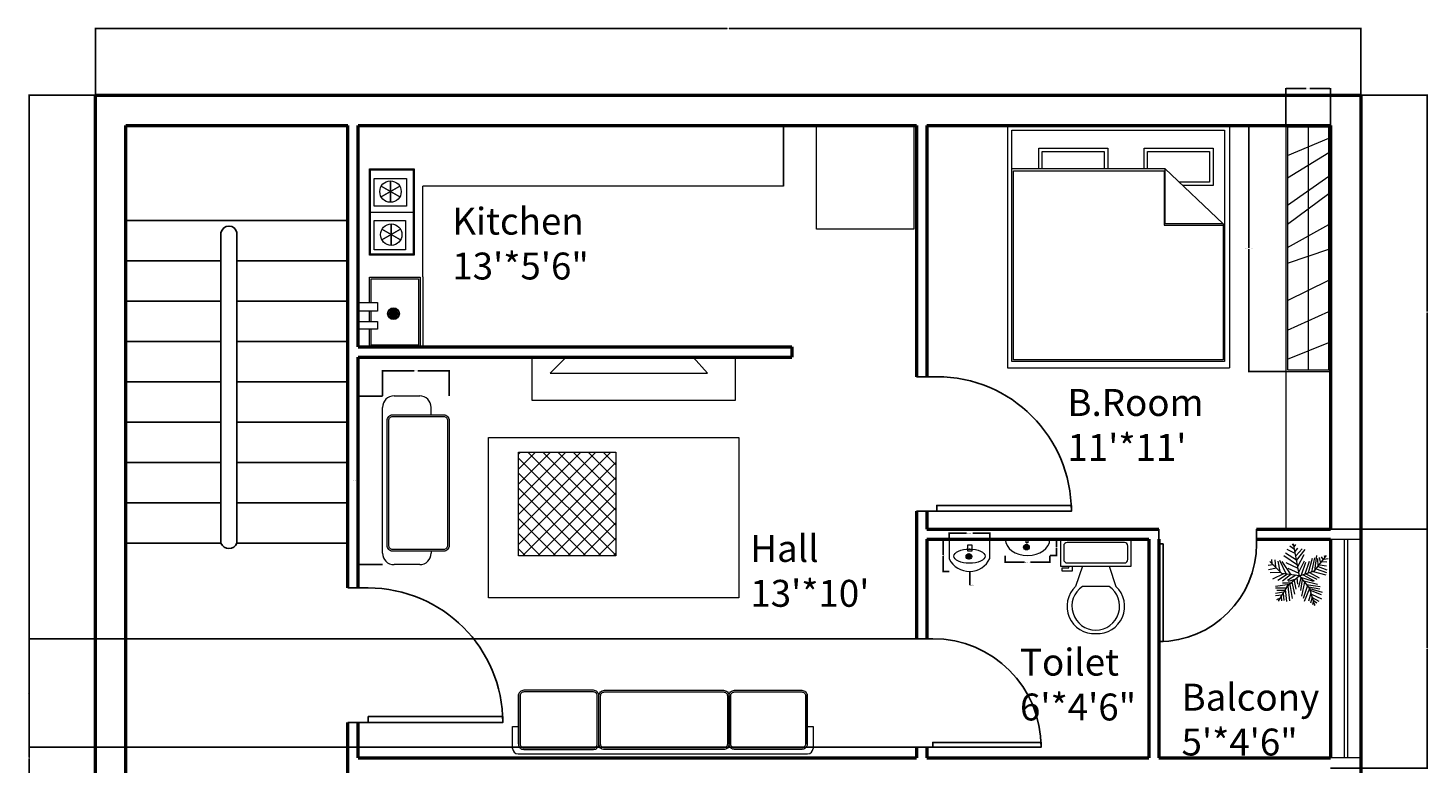
# Model space of a CAD drawing. Units: inches. Extents: x 132738 to 133154, y 138207 to 138641.
# Tile 2 of 2: x 132738 to 133154, y 138422 to 138641. Entities that reach past the tile are written whole.
import ezdxf

# ---------------------------------------------------------------- set-up
doc = ezdxf.new("R2010")
doc.units = ezdxf.units.IN
for name, color, linetype, lineweight in [('A-ANNO-DIMS', 2, 'Continuous', 18), ('A-AREA-IDEN', 7, 'Continuous', 18), ('A-DOOR', 4, 'Continuous', 25), ('A-EQPM', 9, 'Continuous', 18), ('A-FLOR-CASE', 32, 'Continuous', 20), ('A-FLOR-FIXT', 9, 'Continuous', 18), ('A-FLOR-STRS', 7, 'Continuous', 25), ('A-FURN', 8, 'Continuous', 18), ('A-FURN-PATT', 252, 'Continuous', 13), ('A-GLAZ', 4, 'Continuous', 18), ('A-WALL', 7, 'Continuous', 50), ('L-PLNT', 3, 'Continuous', 13)]:
    doc.layers.add(name, color=color, linetype=linetype, lineweight=lineweight)
doc.styles.get("Standard").update_dxf_attribs({"font": 'arial.ttf'})
doc.dimstyles.get("Standard").update_dxf_attribs({"dimtxt": 0.18, "dimasz": 0.18, "dimexe": 0.18, "dimexo": 0.0625, "dimgap": 0.09, "dimtad": 0, "dimtih": 1, "dimtoh": 1, "dimdec": 4, "dimzin": 0, "dimdsep": 46, "dimtxsty": 'Standard', "dimcen": 0.09, "dimadec": 0, "dimazin": 0, "dimtfac": 1, "dimtdec": 4, "dimtofl": 0, "dimtmove": 0, "dimatfit": 3, "dimfxl": 1, "dimtolj": 1, "dimtzin": 0, "dimarcsym": 0})

# ---------------------------------------------------------------- blocks, each defined once
blk = doc.blocks.new('*U4')
for p, q in [((9.5, -6), (9.5, -2)), ((-8, -8.5), (-8, -8)), ((-7, -8), (-7, -9.5)), ((-4, -8), (-6, -14)), ((4, -8), (6, -14)), ((-10, -8.5), (-8, -8.5)), ((-10, -9.5), (-10, -8.5)), ((-7, -9.5), (-10, -9.5)), ((4, -14), (-4, -14))]:
    blk.add_line(p, q)
blk.add_lwpolyline([(10.5, -8), (10.5, 0), (-10.5, 0), (-10.5, -8)], close=True)
for points in [[(-9.5, -2), (-9.5, -6)], [(8.5, -1), (-8.5, -1)], [(-8.5, -7), (8.5, -7)]]:
    blk.add_lwpolyline(points)
for centre, radius, start, end in [((-8.625, -1.875), 0.8839, 81.8699, 188.1301), ((8.625, -1.875), 0.8839, 351.8699, 98.1301), ((-8.625, -6.125), 0.8839, 171.869898, 278.1301), ((8.625, -6.125), 0.8839, 261.8699, 8.1301), ((-0.4772, -19.9188), 8.0953, 133.01722, 273.38), ((0.0374, -19.8731), 7.127, 124.50543, 269.7), ((-0.0373, -19.8731), 7.127, 270.3, 55.4946), ((0.4773, -19.9188), 8.0953, 266.62, 46.9828)]:
    blk.add_arc(centre, radius, start, end)
blk = doc.blocks.new('*U6')
for p, q in [((-8.737, 47.138), (-17.069, 52.711)), ((-10.186, 53.64), (-13.084, 55.962)), ((0, 0), (-10.5, 57)), ((-9.099, 51.782), (-6.563, 55.962)), ((-31.5, 4.5), (-52.5, 25.5)), ((-48.585, 21.131), (-49.309, 29.026)), ((-43.513, 28.561), (-42.427, 15.558)), ((-38.442, 26.239), (-34.819, 7.663)), ((-35.544, 28.097), (-24.314, 3.947)), ((-14.533, 2.09), (-30.834, 25.31)), ((-3.665, 19.273), (-27.574, 35.527)), ((-5.114, 28.097), (-24.676, 40.636)), ((-7.288, 39.707), (-21.778, 46.673)), ((-7.65, 43.423), (-2.578, 49.46)), ((-5.839, 35.992), (4.667, 48.067)), ((-5.114, 27.632), (10.463, 46.673)), ((-2.941, 16.486), (8.652, 37.85)), ((-1.129, 6.734), (9.014, 26.704)), ((10.101, 3.483), (17.708, 26.239)), ((16.259, 5.805), (23.142, 31.348)), ((22.055, 7.198), (27.489, 32.277)), ((27, 9), (48, 36)), ((27.127, 9.056), (31.112, 35.992)), ((31.836, 30.883), (32.561, 16.486)), ((35.096, 32.741), (37.27, 22.524)), ((38.719, 34.134), (41.979, 28.561)), ((40.53, 25.775), (48.862, 24.846)), ((43.791, 29.954), (51.036, 30.883)), ((44.153, 36.456), (45.239, 32.741)), ((-47.498, 19.737), (-55.83, 18.344)), ((-40.615, 13.7), (-55.105, 10.913)), ((-33.37, 6.269), (-52.207, 5.34)), ((-28.299, 3.483), (-47.86, -5.805)), ((-21.416, 3.018), (-38.079, -8.128)), ((0, 0), (-31.5, 4.5)), ((-15.982, 2.09), (-30.11, -9.521)), ((-24.314, 23.917), (-2.941, 13.7)), ((0, 0), (-22.5, -19.5)), ((-6.563, 1.161), (-21.416, -8.128)), ((-20.691, 13.7), (-1.129, 4.876)), ((0, 0), (27, 9)), ((0, 0), (18, -22.5)), ((3.942, 1.625), (11.187, 24.381)), ((6.478, 1.625), (26.04, -8.592)), ((11.187, 3.483), (30.749, -5.805)), ((18.07, 5.805), (35.096, -3.483)), ((24.229, 7.663), (46.688, 1.625)), ((29.662, 12.307), (48.137, 6.269)), ((33.285, 16.486), (48.862, 10.913)), ((36.183, 19.737), (48.137, 17.88)), ((-17.431, -15.094), (-42.789, -18.809)), ((-24.314, -21.596), (-42.427, -22.06)), ((-22.5, -19.5), (-37.5, -45)), ((-15.257, -12.772), (-30.11, -12.772)), ((-25.038, -23.918), (-22.865, -45.281)), ((-20.691, -18.345), (-17.793, -44.352)), ((-6.563, -5.805), (-19.967, -9.985)), ((-17.069, -15.094), (-12.721, -40.172)), ((-13.446, -11.378), (-8.737, -32.741)), ((-9.461, -8.592), (-6.201, -23.453)), ((-4.752, -3.483), (-3.665, -14.629)), ((2.493, -3.019), (-1.491, -20.202)), ((1.769, -2.555), (24.229, -9.521)), ((5.029, -6.27), (2.131, -25.775)), ((9.014, -11.378), (3.58, -35.992)), ((14.085, -16.951), (6.478, -40.172)), ((7.565, -9.056), (32.198, -14.629)), ((18.07, -22.524), (8.289, -45.745)), ((12.274, -15.094), (36.907, -18.809)), ((16.259, -19.738), (36.183, -22.989)), ((18, -22.5), (27, -52.5)), ((18.433, -22.524), (40.53, -29.026)), ((-28.299, -29.026), (-42.789, -31.348)), ((-30.834, -34.135), (-42.427, -35.528)), ((-34.457, -39.708), (-40.978, -42.494)), ((-26.849, -26.24), (-40.253, -25.775)), ((-32.646, -36.921), (-31.921, -44.352)), ((-29.023, -30.884), (-27.936, -43.887)), ((20.244, -30.419), (15.897, -44.816)), ((19.157, -25.311), (38.719, -33.206)), ((22.78, -37.85), (19.519, -48.532)), ((21.331, -32.741), (39.081, -40.636)), ((22.78, -38.314), (34.372, -44.816)), ((24.591, -45.745), (23.142, -50.854)), ((24.591, -43.423), (30.749, -47.603)), ((26.764, -49.925), (28.213, -50.854))]:
    blk.add_line(p, q)
blk = doc.blocks.new('*U2')
for p, q in [((0, 0), (0, -6)), ((40, 0), (40, -6))]:
    blk.add_line(p, q)
blk.add_lwpolyline([(0, 0), (0, 40), (1.75, 40), (1.75, 0)], close=True)
blk.add_arc((0, 0), 40, 0, 90)
blk = doc.blocks.new('SOFA-THREE-SEAT')
for p, q in [((1.73, 2.94), (1.73, 17.66)), ((87.55, 2.94), (87.55, 17.66)), ((87.55, 9.49), (87.55, 8.16)), ((0, 1.62), (0, 8.16)), ((0, 8.16), (1.73, 8.16)), ((87.55, 8.16), (89.29, 8.16)), ((89.29, 8.16), (89.29, 1.62)), ((1.62, 0), (87.67, 0))]:
    blk.add_line(p, q)
for points in [[(3.35, 1.32), (24.03, 1.32, 0.414214), (25.65, 2.94), (25.65, 17.29, 0.414214), (24.03, 18.91), (3.35, 18.91, 0.414214), (1.73, 17.29), (1.73, 2.94, 0.414214)], [(3.35, 1.82), (24.03, 1.82, 0.414214), (25.15, 2.94), (25.15, 17.29, 0.414214), (24.03, 18.41), (3.35, 18.41, 0.414214), (2.23, 17.29), (2.23, 2.94, 0.414214)], [(62.71, 1.26), (27.29, 1.26, -0.414214), (25.67, 2.88), (25.67, 17.29, -0.414214), (27.29, 18.91), (62.71, 18.91, -0.414214), (64.33, 17.29), (64.33, 2.88, -0.414214)], [(62.71, 1.76), (27.29, 1.76, -0.414214), (26.17, 2.88), (26.17, 17.29, -0.414214), (27.29, 18.41), (62.71, 18.41, -0.414214), (63.83, 17.29), (63.83, 2.88, -0.414214)], [(85.93, 1.32), (65.95, 1.32, -0.414214), (64.33, 2.94), (64.33, 17.29, -0.414214), (65.95, 18.91), (85.93, 18.91, -0.414214), (87.55, 17.29), (87.55, 2.94, -0.414214)], [(85.93, 1.82), (65.95, 1.82, -0.414214), (64.83, 2.94), (64.83, 17.29, -0.414214), (65.95, 18.41), (85.93, 18.41, -0.414214), (87.05, 17.29), (87.05, 2.94, -0.414214)]]:
    blk.add_lwpolyline(points, format="xyb", close=True)
for centre, start, end in [((1.62, 1.62), 180, 270), ((87.67, 1.62), 270, 0)]:
    blk.add_arc(centre, 1.62, start, end)
blk = doc.blocks.new('LOUNGE-CHAIR')
for p, q in [((11.02, 50.13), (3.4, 50.13)), ((0, 3.4), (0, 46.74)), ((14.42, 44.54), (14.42, 46.74)), ((14.42, 4.01), (14.42, 3.4)), ((11.02, 0), (3.4, 0))]:
    blk.add_line(p, q)
for points in [[(1.32, 5.71), (1.32, 42.84, -0.414214), (3.02, 44.54), (18.12, 44.54, -0.414214), (19.82, 42.84), (19.82, 5.71, -0.414214), (18.12, 4.01), (3.02, 4.01, -0.414214)], [(1.82, 5.71), (1.82, 42.84, -0.414214), (3.02, 44.04), (18.12, 44.04, -0.414214), (19.32, 42.84), (19.32, 5.71, -0.414214), (18.12, 4.51), (3.02, 4.51, -0.414214)]]:
    blk.add_lwpolyline(points, format="xyb", close=True)
for centre, start, end in [((3.4, 46.74), 90, 180), ((11.02, 46.74), 0, 90), ((3.4, 3.4), 180, 270), ((11.02, 3.4), 270, 0)]:
    blk.add_arc(centre, 3.4, start, end)
blk = doc.blocks.new('*U18')
blk.add_line((0, 6.36), (0, 0))
blk = doc.blocks.new('*U19')
at = {"color": 0, "linetype": 'ByBlock', "lineweight": -2, "transparency": 16777216}
for p, rotation in [((132078.56, 137807.89), 59.99999999999997), ((132078.56, 137811.07), 119.9999999999999), ((132073.05, 137811.07), 240), ((132073.05, 137807.89), 300), ((132075.81, 137812.66), 180)]:
    blk.add_blockref('*U18', p, dxfattribs=dict(at, rotation=rotation))
blk.add_blockref('*U18', (132075.81, 137806.3), dxfattribs=at)
blk = doc.blocks.new('*U20')
blk.add_line((0, 6.36), (0, 0))
blk = doc.blocks.new('*U21')
at = {"color": 0, "linetype": 'ByBlock', "lineweight": -2, "transparency": 16777216}
for p, rotation in [((132078.34, 137820.7), 59.99999999999997), ((132078.34, 137823.88), 119.9999999999999), ((132072.84, 137823.88), 240), ((132072.84, 137820.7), 300), ((132075.59, 137825.47), 180)]:
    blk.add_blockref('*U20', p, dxfattribs=dict(at, rotation=rotation))
blk.add_blockref('*U20', (132075.59, 137819.12), dxfattribs=at)
blk = doc.blocks.new('COOKTOP-TWO-BURNER')
blk.add_line((0, 12.86), (13.26, 12.86))
for points in [[(0, 25.73), (13.26, 25.73), (13.26, 0), (0, 0)], [(0.3, 25.43), (12.96, 25.43), (12.96, 0.3), (0.3, 0.3)], [(1.41, 22.8), (10.98, 22.8), (10.98, 14.61), (1.41, 14.61)], [(1.41, 10.35), (10.68, 10.35), (10.68, 1.58), (1.41, 1.58)]]:
    blk.add_lwpolyline(points, close=True)
for centre in [(6.25, 18.94), (6.47, 6.13)]:
    blk.add_circle(centre, 3.18)
for name in ['*U21', '*U19']:
    blk.add_blockref(name, (-132069.34, -137803.35))
blk = doc.blocks.new('*U16')
blk.add_line((0, 3.48), (0, 0))
blk = doc.blocks.new('*U17')
at = {"color": 0, "linetype": 'ByBlock', "lineweight": -2, "transparency": 16777216}
for p, rotation in [((132078.13, 137785.45), 71.99999999999999), ((132078.13, 137786.53), 108), ((132074.83, 137786.53), 252), ((132074.83, 137785.45), 288), ((132077.89, 137784.97), 53.99999999999998), ((132077.89, 137787.01), 126), ((132075.08, 137787.01), 234), ((132075.08, 137784.97), 306), ((132077.5, 137784.59), 35.99999999999999), ((132077.5, 137787.4), 144), ((132075.46, 137787.4), 216), ((132075.46, 137784.59), 323.9999999999999), ((132077.02, 137784.34), 17.99999999999998), ((132077.02, 137787.64), 162), ((132075.95, 137787.64), 198), ((132075.95, 137784.34), 342), ((132076.48, 137787.73), 180), ((132078.22, 137785.99), 90), ((132074.74, 137785.99), 270)]:
    blk.add_blockref('*U16', p, dxfattribs=dict(at, rotation=rotation))
blk.add_blockref('*U16', (132076.48, 137784.25), dxfattribs=at)
blk = doc.blocks.new('SINK-KITCHEN')
blk.add_line((3.38, 20.8), (18.5, 20.8))
for points in [[(3.38, 13.25), (3.38, 20.8), (18.5, 20.8), (18.5, 0), (3.38, 0), (3.38, 5.25)], [(3.88, 13.25), (3.88, 20.3), (18, 20.3), (18, 0.5), (3.88, 0.5), (3.88, 5.25)], [(3.38, 7.61), (3.38, 10.65)], [(3.88, 7.61), (3.88, 10.65)]]:
    blk.add_lwpolyline(points)
for points in [[(0, 13.25), (5.74, 13.25), (5.74, 10.65), (0, 10.65)], [(0, 7.61), (5.74, 7.61), (5.74, 5.25), (0, 5.25)]]:
    blk.add_lwpolyline(points, close=True)
blk.add_circle((10.52, 9.9), 1.74)
blk.add_blockref('*U17', (-132065.96, -137776.09))
blk = doc.blocks.new('*U9')
blk.add_line((0, 1.68), (0, 0))
blk = doc.blocks.new('*U10')
at = {"color": 0, "linetype": 'ByBlock', "lineweight": -2, "transparency": 16777216}
for p, rotation in [((132265.47, 137716.61), 90), ((132263.79, 137716.61), 270), ((132265.42, 137716.35), 71.99999999999999), ((132265.42, 137716.87), 108), ((132263.83, 137716.87), 252), ((132263.83, 137716.35), 288), ((132265.31, 137716.12), 53.99999999999998), ((132265.31, 137717.1), 126), ((132263.95, 137717.1), 234), ((132263.95, 137716.12), 306), ((132265.12, 137715.93), 35.99999999999999), ((132265.12, 137717.29), 144), ((132264.13, 137717.29), 216), ((132264.13, 137715.93), 324), ((132264.89, 137715.81), 17.99999999999997), ((132264.89, 137717.41), 162), ((132264.37, 137717.41), 197.9999999999999), ((132264.37, 137715.81), 342), ((132264.63, 137717.45), 180)]:
    blk.add_blockref('*U9', p, dxfattribs=dict(at, rotation=rotation))
blk.add_blockref('*U9', (132264.63, 137715.77), dxfattribs=at)
blk = doc.blocks.new('BASIN-OVAL')
blk.add_lwpolyline([(6.22, 4.85), (6.68, 4.85), (6.68, 3.77), (6.22, 3.77)], close=True)
blk.add_circle((6.31, 2.53), 0.838)
blk.add_ellipse((6.62, 4.85), major_axis=(6.62, 0), ratio=0.732474, start_param=3.141593, end_param=6.283185)
blk.add_blockref('*U10', (-132258.32, -137714.08))
blk = doc.blocks.new('*U11')
blk.add_line((0, 1.68), (0, 0))
blk = doc.blocks.new('*U12')
at = {"color": 0, "linetype": 'ByBlock', "lineweight": -2, "transparency": 16777216}
for p, rotation in [((132265.47, 137716.61), 90), ((132263.79, 137716.61), 270), ((132265.42, 137716.35), 71.99999999999999), ((132265.42, 137716.87), 108), ((132263.83, 137716.87), 252), ((132263.83, 137716.35), 288), ((132265.31, 137716.12), 53.99999999999998), ((132265.31, 137717.1), 126), ((132263.95, 137717.1), 234), ((132263.95, 137716.12), 306), ((132265.12, 137715.93), 35.99999999999999), ((132265.12, 137717.29), 144), ((132264.13, 137717.29), 216), ((132264.13, 137715.93), 324), ((132264.89, 137715.81), 17.99999999999997), ((132264.89, 137717.41), 162), ((132264.37, 137717.41), 197.9999999999999), ((132264.37, 137715.81), 342), ((132264.63, 137717.45), 180)]:
    blk.add_blockref('*U11', p, dxfattribs=dict(at, rotation=rotation))
blk.add_blockref('*U11', (132264.63, 137715.77), dxfattribs=at)
blk = doc.blocks.new('BASIN-WALL')
for p, q in [((0, 9.56), (0, 3.71)), ((12.04, 3.88), (12.04, 9.56))]:
    blk.add_line(p, q)
blk.add_lwpolyline([(5.55, 7.94), (6.68, 7.94), (6.68, 6.05), (5.55, 6.05)], close=True)
blk.add_circle((5.81, 4.48), 0.838)
blk.add_arc((5.98, 6.67), 6.67, 206.3567, 335.2907)
blk.add_ellipse((5.98, 4.55), major_axis=(4.63, 0), ratio=0.457552)
blk.add_blockref('*U12', (-132258.82, -137712.13))
blk = doc.blocks.new('BED-DOUBLE')
for p, q in [((0, 72), (0, 0)), ((66, 72), (66, 0)), ((1.29, 59.19), (46.8, 59.19)), ((46.61, 58.57), (46.61, 42.39)), ((46.8, 59.19), (64.12, 42.79)), ((46.8, 59.19), (46.8, 42.79)), ((46.61, 42.39), (64.12, 42.39)), ((64.12, 42.79), (46.8, 42.79)), ((0, 0), (66, 0))]:
    blk.add_line(p, q)
blk.add_lwpolyline([(1.29, 70.58), (64.54, 70.58), (64.54, 1.81), (1.29, 1.81)], close=True)
blk.add_lwpolyline([(64.12, 42.79), (64.12, 2.3), (1.76, 2.3), (1.76, 58.57), (46.61, 58.57)])
blk = doc.blocks.new('WARDROBE')
for p, q in [((6.65, 72.63), (6.65, 0.5)), ((0.5, 64.18), (12.79, 69.35)), ((0.5, 57.53), (12.79, 65.06)), ((0.5, 49.42), (12.79, 58.04)), ((0.5, 43.85), (12.79, 52.9)), ((0.5, 36.84), (12.79, 43.67)), ((0.5, 32.25), (12.79, 36.4)), ((0.5, 21.15), (12.79, 27.18)), ((0.5, 12.28), (12.79, 17.88)), ((0.5, 3.64), (12.79, 8.6))]:
    blk.add_line(p, q)
for points in [[(13.29, 73.13), (0, 73.13), (0, 0), (13.29, 0)], [(12.79, 72.63), (0.5, 72.63), (0.5, 0.5), (12.79, 0.5)]]:
    blk.add_lwpolyline(points, close=True)
blk = doc.blocks.new('TV-FLATSCREEN')
for p, q in [((4.76, 4.76), (0, 0)), ((46.75, 0), (42.54, 4.76)), ((0, 0), (46.75, 0))]:
    blk.add_line(p, q)
blk = doc.blocks.new('*D36')
at = {"layer": 'A-ANNO-DIMS', "color": 0, "lineweight": -2, "transparency": 16777216}
for p, q in [((132843.18, 138531.51), (132835.55, 138531.51)), ((132835.73, 138531.33), (132835.73, 138506.63)), ((132835.73, 138481.56), (132835.73, 138506.26)), ((132843.18, 138481.38), (132835.55, 138481.38))]:
    blk.add_line(p, q, dxfattribs=at)
at = {"layer": 'A-ANNO-DIMS', "color": 0, "transparency": 16777216}
for points in [[(132835.7, 138531.33), (132835.76, 138531.33), (132835.73, 138531.51)], [(132835.7, 138481.56), (132835.76, 138481.56), (132835.73, 138481.38)]]:
    blk.add_solid(points, dxfattribs=at)
at = {"layer": 'Defpoints', "color": 0, "transparency": 16777216}
for p in [(132835.73, 138531.51), (132843.25, 138531.51), (132843.25, 138481.38)]:
    blk.add_point(p, dxfattribs=at)
at = {"layer": 'A-ANNO-DIMS', "color": 0, "transparency": 16777216, "insert": (132835.73, 138506.45), "char_height": 0.18, "attachment_point": 5}
blk.add_mtext('\\A1;LOUNGE CHAIR 50 TYP.', dxfattribs=at)
blk = doc.blocks.new('*D37')
at = {"layer": 'A-ANNO-DIMS', "color": 0, "lineweight": -2, "transparency": 16777216}
for p, q in [((132843.25, 138531.58), (132843.25, 138539.21)), ((132843.43, 138539.03), (132852.63, 138539.03)), ((132862.89, 138539.03), (132853.69, 138539.03)), ((132863.07, 138531.58), (132863.07, 138539.21))]:
    blk.add_line(p, q, dxfattribs=at)
at = {"layer": 'A-ANNO-DIMS', "color": 0, "transparency": 16777216}
for points in [[(132843.43, 138539.06), (132843.43, 138539), (132843.25, 138539.03)], [(132862.89, 138539.06), (132862.89, 138539), (132863.07, 138539.03)]]:
    blk.add_solid(points, dxfattribs=at)
at = {"layer": 'Defpoints', "color": 0, "transparency": 16777216}
for p in [(132863.07, 138539.03), (132843.25, 138531.51), (132863.07, 138531.51)]:
    blk.add_point(p, dxfattribs=at)
at = {"layer": 'A-ANNO-DIMS', "color": 0, "transparency": 16777216, "insert": (132853.16, 138539.03), "char_height": 0.18, "attachment_point": 5}
blk.add_mtext('\\A1;20 TYP.', dxfattribs=at)
blk = doc.blocks.new('*D42')
at = {"layer": 'A-ANNO-DIMS', "color": 0, "lineweight": -2, "transparency": 16777216}
for p, q in [((133028.32, 138484.01), (133028.32, 138481.91)), ((133028.5, 138482.09), (133034.04, 138482.09)), ((133041.37, 138482.09), (133035.83, 138482.09)), ((133041.55, 138484.01), (133041.55, 138481.91))]:
    blk.add_line(p, q, dxfattribs=at)
at = {"layer": 'A-ANNO-DIMS', "color": 0, "transparency": 16777216}
for points in [[(133028.5, 138482.12), (133028.5, 138482.06), (133028.32, 138482.09)], [(133041.37, 138482.12), (133041.37, 138482.06), (133041.55, 138482.09)]]:
    blk.add_solid(points, dxfattribs=at)
at = {"layer": 'Defpoints', "color": 0, "transparency": 16777216}
for p in [(133028.32, 138484.08), (133041.55, 138484.08), (133041.55, 138482.09)]:
    blk.add_point(p, dxfattribs=at)
at = {"layer": 'A-ANNO-DIMS', "color": 0, "transparency": 16777216, "insert": (133034.94, 138482.09), "char_height": 0.18, "attachment_point": 5}
blk.add_mtext('\\A1;OVAL 13 TYP.', dxfattribs=at)
blk = doc.blocks.new('*D43')
at = {"layer": 'A-ANNO-DIMS', "color": 0, "lineweight": -2, "transparency": 16777216}
for p, q in [((133041.62, 138488.92), (133043.72, 138488.92)), ((133043.54, 138488.74), (133043.54, 138486.68)), ((133043.54, 138484.26), (133043.54, 138486.32)), ((133041.62, 138484.08), (133043.72, 138484.08))]:
    blk.add_line(p, q, dxfattribs=at)
at = {"layer": 'A-ANNO-DIMS', "color": 0, "transparency": 16777216}
for points in [[(133043.51, 138488.74), (133043.57, 138488.74), (133043.54, 138488.92)], [(133043.51, 138484.26), (133043.57, 138484.26), (133043.54, 138484.08)]]:
    blk.add_solid(points, dxfattribs=at)
at = {"layer": 'Defpoints', "color": 0, "transparency": 16777216}
for p in [(133041.55, 138488.92), (133043.54, 138488.92), (133041.55, 138484.08)]:
    blk.add_point(p, dxfattribs=at)
at = {"layer": 'A-ANNO-DIMS', "color": 0, "transparency": 16777216, "insert": (133043.54, 138486.5), "char_height": 0.18, "attachment_point": 5}
blk.add_mtext('\\A1;5 TYP.', dxfattribs=at)
blk = doc.blocks.new('*D44')
at = {"layer": 'A-ANNO-DIMS', "color": 0, "lineweight": -2, "transparency": 16777216}
for p, q in [((133011.69, 138488.99), (133011.69, 138490.91)), ((133011.87, 138490.73), (133016.77, 138490.73)), ((133023.55, 138490.73), (133018.65, 138490.73)), ((133023.73, 138488.99), (133023.73, 138490.91))]:
    blk.add_line(p, q, dxfattribs=at)
at = {"layer": 'A-ANNO-DIMS', "color": 0, "transparency": 16777216}
for points in [[(133011.87, 138490.76), (133011.87, 138490.7), (133011.69, 138490.73)], [(133023.55, 138490.76), (133023.55, 138490.7), (133023.73, 138490.73)]]:
    blk.add_solid(points, dxfattribs=at)
at = {"layer": 'Defpoints', "color": 0, "transparency": 16777216}
for p in [(133023.73, 138490.73), (133011.69, 138488.92), (133023.73, 138488.92)]:
    blk.add_point(p, dxfattribs=at)
at = {"layer": 'A-ANNO-DIMS', "color": 0, "transparency": 16777216, "insert": (133017.71, 138490.73), "char_height": 0.18, "attachment_point": 5}
blk.add_mtext('\\A1;BASIN 12 TYP.', dxfattribs=at)
blk = doc.blocks.new('*D45')
at = {"layer": 'A-ANNO-DIMS', "color": 0, "lineweight": -2, "transparency": 16777216}
for p, q in [((133011.63, 138488.92), (133009.7, 138488.92)), ((133009.88, 138488.74), (133009.88, 138484.31)), ((133009.88, 138479.5), (133009.88, 138483.94)), ((133011.63, 138479.32), (133009.7, 138479.32))]:
    blk.add_line(p, q, dxfattribs=at)
at = {"layer": 'A-ANNO-DIMS', "color": 0, "transparency": 16777216}
for points in [[(133009.85, 138488.74), (133009.91, 138488.74), (133009.88, 138488.92)], [(133009.85, 138479.5), (133009.91, 138479.5), (133009.88, 138479.32)]]:
    blk.add_solid(points, dxfattribs=at)
at = {"layer": 'Defpoints', "color": 0, "transparency": 16777216}
for p in [(133009.88, 138488.92), (133011.69, 138488.92), (133011.69, 138479.32)]:
    blk.add_point(p, dxfattribs=at)
at = {"layer": 'A-ANNO-DIMS', "color": 0, "transparency": 16777216, "insert": (133009.88, 138484.12), "char_height": 0.18, "attachment_point": 5}
blk.add_mtext('\\A1;10 TYP.', dxfattribs=at)
blk = doc.blocks.new('*D48')
at = {"layer": 'A-ANNO-DIMS', "color": 0, "lineweight": -2, "transparency": 16777216}
for p, q in [((133111.6, 138611.92), (133100.52, 138611.92)), ((133100.7, 138611.74), (133100.7, 138575.54)), ((133100.7, 138538.97), (133100.7, 138575.17)), ((133111.6, 138538.79), (133100.52, 138538.79))]:
    blk.add_line(p, q, dxfattribs=at)
at = {"layer": 'A-ANNO-DIMS', "color": 0, "transparency": 16777216}
for points in [[(133100.67, 138611.74), (133100.73, 138611.74), (133100.7, 138611.92)], [(133100.67, 138538.97), (133100.73, 138538.97), (133100.7, 138538.79)]]:
    blk.add_solid(points, dxfattribs=at)
at = {"layer": 'Defpoints', "color": 0, "transparency": 16777216}
for p in [(133100.7, 138611.92), (133111.67, 138611.92), (133111.67, 138538.79)]:
    blk.add_point(p, dxfattribs=at)
at = {"layer": 'A-ANNO-DIMS', "color": 0, "transparency": 16777216, "insert": (133100.7, 138575.36), "char_height": 0.18, "attachment_point": 5}
blk.add_mtext('\\A1;WARDROBE 73 TYP.', dxfattribs=at)
blk = doc.blocks.new('*D49')
at = {"layer": 'A-ANNO-DIMS', "color": 0, "lineweight": -2, "transparency": 16777216}
for p, q in [((133111.67, 138611.99), (133111.67, 138623.07)), ((133111.85, 138622.89), (133117.79, 138622.89)), ((133124.78, 138622.89), (133118.83, 138622.89)), ((133124.96, 138611.99), (133124.96, 138623.07))]:
    blk.add_line(p, q, dxfattribs=at)
at = {"layer": 'A-ANNO-DIMS', "color": 0, "transparency": 16777216}
for points in [[(133111.85, 138622.92), (133111.85, 138622.86), (133111.67, 138622.89)], [(133124.78, 138622.92), (133124.78, 138622.86), (133124.96, 138622.89)]]:
    blk.add_solid(points, dxfattribs=at)
at = {"layer": 'Defpoints', "color": 0, "transparency": 16777216}
for p in [(133124.96, 138622.89), (133111.67, 138611.92), (133124.96, 138611.92)]:
    blk.add_point(p, dxfattribs=at)
at = {"layer": 'A-ANNO-DIMS', "color": 0, "transparency": 16777216, "insert": (133118.31, 138622.89), "char_height": 0.18, "attachment_point": 5}
blk.add_mtext('\\A1;13 TYP.', dxfattribs=at)
blk = doc.blocks.new('*D52')
at = {"layer": 'A-ANNO-DIMS', "color": 0, "lineweight": -2, "transparency": 16777216}
for p, q in [((132757.96, 138620.99), (132757.96, 138640.91)), ((132758.14, 138640.73), (132945.67, 138640.73)), ((133133.78, 138640.73), (132946.25, 138640.73)), ((133133.96, 138620.99), (133133.96, 138640.91))]:
    blk.add_line(p, q, dxfattribs=at)
at = {"layer": 'A-ANNO-DIMS', "color": 0, "transparency": 16777216}
for points in [[(132758.14, 138640.76), (132758.14, 138640.7), (132757.96, 138640.73)], [(133133.78, 138640.76), (133133.78, 138640.7), (133133.96, 138640.73)]]:
    blk.add_solid(points, dxfattribs=at)
at = {"layer": 'Defpoints', "color": 0, "transparency": 16777216}
for p in [(133133.96, 138640.73), (132757.96, 138620.92), (133133.96, 138620.92)]:
    blk.add_point(p, dxfattribs=at)
at = {"layer": 'A-ANNO-DIMS', "color": 0, "transparency": 16777216, "insert": (132945.96, 138640.73), "char_height": 0.18, "attachment_point": 5}
blk.add_mtext('\\A1;376', dxfattribs=at)
blk = doc.blocks.new('*D53')
at = {"layer": 'A-ANNO-DIMS', "color": 0, "lineweight": -2, "transparency": 16777216}
for p, q in [((132757.9, 138620.92), (132737.98, 138620.92)), ((132738.16, 138620.74), (132738.16, 138424.1)), ((132738.16, 138227.1), (132738.16, 138423.74)), ((132757.9, 138226.92), (132737.98, 138226.92))]:
    blk.add_line(p, q, dxfattribs=at)
at = {"layer": 'A-ANNO-DIMS', "color": 0, "transparency": 16777216}
for points in [[(132738.13, 138620.74), (132738.19, 138620.74), (132738.16, 138620.92)], [(132738.13, 138227.1), (132738.19, 138227.1), (132738.16, 138226.92)]]:
    blk.add_solid(points, dxfattribs=at)
at = {"layer": 'Defpoints', "color": 0, "transparency": 16777216}
for p in [(132738.16, 138620.92), (132757.96, 138620.92), (132757.96, 138226.92)]:
    blk.add_point(p, dxfattribs=at)
at = {"layer": 'A-ANNO-DIMS', "color": 0, "transparency": 16777216, "insert": (132738.16, 138423.92), "char_height": 0.18, "attachment_point": 5}
blk.add_mtext('\\A1;394', dxfattribs=at)
blk = doc.blocks.new('*D60')
at = {"layer": 'A-ANNO-DIMS', "color": 0, "lineweight": -2, "transparency": 16777216}
for p, q in [((133001.9, 138459.36), (132737.98, 138459.36)), ((132738.16, 138459.18), (132738.16, 138443.44)), ((132738.16, 138427.33), (132738.16, 138443.08)), ((133001.9, 138427.15), (132737.98, 138427.15))]:
    blk.add_line(p, q, dxfattribs=at)
at = {"layer": 'A-ANNO-DIMS', "color": 0, "transparency": 16777216}
for points in [[(132738.13, 138459.18), (132738.19, 138459.18), (132738.16, 138459.36)], [(132738.13, 138427.33), (132738.19, 138427.33), (132738.16, 138427.15)]]:
    blk.add_solid(points, dxfattribs=at)
at = {"layer": 'Defpoints', "color": 0, "transparency": 16777216}
for p in [(132738.16, 138459.36), (133001.96, 138459.36), (133001.96, 138427.15)]:
    blk.add_point(p, dxfattribs=at)
at = {"layer": 'A-ANNO-DIMS', "color": 0, "transparency": 16777216, "insert": (132738.16, 138443.26), "char_height": 0.18, "attachment_point": 5}
blk.add_mtext('\\A1;32.21', dxfattribs=at)
blk = doc.blocks.new('*D61')
at = {"layer": 'A-ANNO-DIMS', "color": 0, "lineweight": -2, "transparency": 16777216}
for p, q in [((133125.02, 138491.92), (133153.95, 138491.92)), ((133153.77, 138491.74), (133153.77, 138456.6)), ((133153.77, 138421.1), (133153.77, 138456.24)), ((133125.02, 138420.92), (133153.95, 138420.92))]:
    blk.add_line(p, q, dxfattribs=at)
at = {"layer": 'A-ANNO-DIMS', "color": 0, "transparency": 16777216}
for points in [[(133153.74, 138491.74), (133153.8, 138491.74), (133153.77, 138491.92)], [(133153.74, 138421.1), (133153.8, 138421.1), (133153.77, 138420.92)]]:
    blk.add_solid(points, dxfattribs=at)
at = {"layer": 'Defpoints', "color": 0, "transparency": 16777216}
for p in [(133124.96, 138491.92), (133153.77, 138491.92), (133124.96, 138420.92)]:
    blk.add_point(p, dxfattribs=at)
at = {"layer": 'A-ANNO-DIMS', "color": 0, "transparency": 16777216, "insert": (133153.77, 138456.42), "char_height": 0.18, "attachment_point": 5}
blk.add_mtext('\\A1;71', dxfattribs=at)
blk = doc.blocks.new('*D62')
at = {"layer": 'A-ANNO-DIMS', "color": 0, "lineweight": -2, "transparency": 16777216}
for p, q in [((133134.02, 138620.92), (133153.95, 138620.92)), ((133153.77, 138620.74), (133153.77, 138556.6)), ((133153.77, 138492.1), (133153.77, 138556.24)), ((133125.02, 138491.92), (133153.95, 138491.92))]:
    blk.add_line(p, q, dxfattribs=at)
at = {"layer": 'A-ANNO-DIMS', "color": 0, "transparency": 16777216}
for points in [[(133153.74, 138620.74), (133153.8, 138620.74), (133153.77, 138620.92)], [(133153.74, 138492.1), (133153.8, 138492.1), (133153.77, 138491.92)]]:
    blk.add_solid(points, dxfattribs=at)
at = {"layer": 'Defpoints', "color": 0, "transparency": 16777216}
for p in [(133133.96, 138620.92), (133153.77, 138620.92), (133124.96, 138491.92)]:
    blk.add_point(p, dxfattribs=at)
at = {"layer": 'A-ANNO-DIMS', "color": 0, "transparency": 16777216, "insert": (133153.77, 138556.42), "char_height": 0.18, "attachment_point": 5}
blk.add_mtext('\\A1;129', dxfattribs=at)
blk = doc.blocks.new('*D63')
at = {"layer": 'A-ANNO-DIMS', "color": 0, "lineweight": -2, "transparency": 16777216}
for p, q in [((133017.58, 138486.03), (133017.76, 138486.03)), ((133017.67, 138485.94), (133017.67, 138486.12)), ((133017.82, 138475.36), (133017.77, 138479.18)), ((133018, 138475.36), (133017.82, 138475.36))]:
    blk.add_line(p, q, dxfattribs=at)
at = {"layer": 'A-ANNO-DIMS', "color": 0, "transparency": 16777216}
blk.add_solid([(133017.8, 138479.18), (133017.74, 138479.18), (133017.76, 138479.36)], dxfattribs=at)
at = {"layer": 'Defpoints', "color": 0, "transparency": 16777216}
for p in [(133017.67, 138486.03), (133017.76, 138479.36)]:
    blk.add_point(p, dxfattribs=at)
at = {"layer": 'A-ANNO-DIMS', "color": 0, "transparency": 16777216, "insert": (133018.61, 138475.36), "char_height": 0.18, "attachment_point": 5}
blk.add_mtext('\\A1;2X R6.67', dxfattribs=at)

msp = doc.modelspace()

# ---------------------------------------------------------------- hatches: boundary and pattern name
at = {"layer": 'A-FURN-PATT'}
h = msp.add_hatch(dxfattribs=at)
h.set_pattern_fill('ANSI37', color=256)
h.set_pattern_definition([(45, (770, 770), (-2.24506403, 2.24506403), []), (135, (770, 770), (-2.24506403, -2.24506403), [])])
h.paths.add_polyline_path([(132883.645, 138514.812), (132912.545, 138514.812), (132912.545, 138484.038), (132883.645, 138484.038)])

# ---------------------------------------------------------------- linework, layer by layer
at = {"layer": 'A-EQPM'}
msp.add_lwpolyline([(132972.224, 138611.923), (133001.124, 138611.923), (133001.124, 138581.149), (132972.224, 138581.149)], close=True, dxfattribs=at)
at = {"layer": 'A-FLOR-CASE'}
for p, q in [((132962.423, 138593.854), (132962.423, 138611.923)), ((132962.423, 138611.923), (132962.423, 138593.854)), ((132855.161, 138566.891), (132855.161, 138593.854)), ((132962.423, 138593.854), (132855.161, 138593.854)), ((132855.161, 138566.891), (132855.161, 138546.088)), ((133111.667, 138538.792), (133111.667, 138491.923))]:
    msp.add_line(p, q, dxfattribs=at)
at = {"layer": 'A-FLOR-STRS'}
for p, q in [((132766.961, 138583.724), (132799.961, 138583.724)), ((132799.961, 138583.724), (132832.961, 138583.724)), ((132766.961, 138571.724), (132795.211, 138571.724)), ((132799.961, 138571.724), (132832.961, 138571.724)), ((132766.961, 138559.724), (132795.211, 138559.724)), ((132799.961, 138559.724), (132832.961, 138559.724)), ((132766.961, 138547.724), (132795.211, 138547.724)), ((132799.961, 138547.724), (132832.961, 138547.724)), ((132766.961, 138535.724), (132795.211, 138535.724)), ((132799.961, 138535.724), (132832.961, 138535.724)), ((132766.961, 138523.724), (132795.211, 138523.724)), ((132799.961, 138523.724), (132832.961, 138523.724)), ((132766.961, 138511.724), (132795.211, 138511.724)), ((132799.961, 138511.724), (132832.961, 138511.724)), ((132766.961, 138499.724), (132795.211, 138499.724)), ((132799.961, 138499.724), (132832.961, 138499.724)), ((132766.961, 138487.724), (132795.211, 138487.724)), ((132799.961, 138487.724), (132832.961, 138487.724))]:
    msp.add_line(p, q, dxfattribs=at)
for points in [[(132795.211, 138487.724), (132795.211, 138580.071)], [(132799.961, 138580.071), (132799.961, 138487.724)]]:
    msp.add_lwpolyline(points, dxfattribs=at)
for centre, radius, start, end in [((132797.586, 138579.601), 2.421, 11.19027, 168.80973), ((132797.586, 138488.779), 2.599, 203.93158, 336.06842)]:
    msp.add_arc(centre, radius, start, end, dxfattribs=at)
at = {"layer": 'A-FURN'}
for points in [[(133038.293, 138599.112), (133038.293, 138605.195), (133058.767, 138605.195), (133058.767, 138599.112)], [(133039.293, 138599.112), (133039.293, 138604.195), (133057.767, 138604.195), (133057.767, 138599.112)], [(133069.6, 138599.112), (133069.6, 138605.195), (133090.073, 138605.195), (133090.073, 138594.072), (133081.081, 138594.072)], [(133070.6, 138599.112), (133070.6, 138604.195), (133089.073, 138604.195), (133089.073, 138595.072), (133080.024, 138595.072)]]:
    msp.add_lwpolyline(points, dxfattribs=at)
for points in [[(132887.751, 138543.088), (132948.088, 138543.088), (132948.088, 138530.19), (132887.751, 138530.19)], [(132874.721, 138519.165), (132949.136, 138519.165), (132949.136, 138471.53), (132874.721, 138471.53)], [(132883.645, 138514.812), (132912.545, 138514.812), (132912.545, 138484.038), (132883.645, 138484.038)]]:
    msp.add_lwpolyline(points, close=True, dxfattribs=at)
at = {"layer": 'A-GLAZ'}
for p, q in [((133129.023, 138488.923), (133129.023, 138423.923)), ((133130.023, 138488.923), (133130.023, 138423.923))]:
    msp.add_line(p, q, dxfattribs=at)
msp.add_lwpolyline([(133124.961, 138488.923), (133133.961, 138488.923), (133133.961, 138423.923), (133124.961, 138423.923)], close=True, dxfattribs=at)
at = {"layer": 'A-WALL'}
for p, q in [((132757.961, 138620.923), (133133.961, 138620.923)), ((132757.961, 138226.923), (132757.961, 138620.923)), ((133133.961, 138620.923), (133133.961, 138226.923)), ((132766.961, 138611.923), (132832.961, 138611.923)), ((132766.961, 138235.923), (132766.961, 138611.923)), ((132832.961, 138474.453), (132832.961, 138611.923)), ((132835.961, 138611.923), (133001.961, 138611.923)), ((132835.961, 138557.923), (132835.961, 138611.923)), ((133001.961, 138611.923), (133001.961, 138557.923)), ((133004.961, 138611.923), (133004.961, 138537.261)), ((133004.961, 138611.923), (133124.961, 138611.923)), ((133124.961, 138611.923), (133124.961, 138491.923)), ((132835.961, 138546.088), (132835.961, 138557.923)), ((133001.961, 138557.923), (133001.961, 138546.088)), ((132835.961, 138546.088), (132964.885, 138546.088)), ((132964.885, 138546.088), (132964.885, 138543.088)), ((133001.961, 138546.088), (133001.961, 138537.261)), ((132835.961, 138543.088), (132964.885, 138543.088)), ((132835.961, 138474.453), (132835.961, 138543.088)), ((133001.961, 138497.261), (133001.961, 138459.361)), ((133004.961, 138497.261), (133004.961, 138491.923)), ((133004.961, 138491.923), (133073.961, 138491.923)), ((133103, 138491.923), (133124.961, 138491.923)), ((133004.961, 138488.923), (133070.961, 138488.923)), ((133004.961, 138488.923), (133004.961, 138459.361)), ((133070.961, 138488.923), (133070.961, 138423.923)), ((133073.961, 138488.923), (133073.961, 138423.923)), ((133103, 138488.923), (133124.961, 138488.923)), ((133124.961, 138488.923), (133124.961, 138423.923)), ((132832.961, 138286.105), (132832.961, 138434.453)), ((132835.961, 138423.923), (132835.961, 138434.453)), ((133001.961, 138427.153), (133001.961, 138423.923)), ((133004.961, 138427.153), (133004.961, 138423.923)), ((132835.961, 138423.923), (133001.961, 138423.923)), ((133004.961, 138423.923), (133070.961, 138423.923)), ((133073.961, 138423.923), (133124.961, 138423.923))]:
    msp.add_line(p, q, dxfattribs=at)

# ---------------------------------------------------------------- block references
at = {"layer": 'A-DOOR', "xscale": -1, "rotation": 270}
for p in [(133007.961, 138497.261), (132838.961, 138434.453)]:
    msp.add_blockref('*U2', p, dxfattribs=at)
at = {"layer": 'A-DOOR'}
for p, xscale, yscale, zscale, rotation in [((133073.961, 138487.567), -0.7259678635176819, 0.7259678635176819, 0.7259678635176819, 180), ((133006.792, 138427.153), -0.8051920827698534, 0.8051920827698534, 0.8051920827698534, 270)]:
    msp.add_blockref('*U2', p, dxfattribs=dict(at, xscale=xscale, yscale=yscale, zscale=zscale, rotation=rotation))
at = {"layer": 'A-EQPM'}
for name, p in [('COOKTOP-TWO-BURNER', (132839.34, 138573.35)), ('TV-FLATSCREEN', (132893.062, 138538.324))]:
    msp.add_blockref(name, p, dxfattribs=at)
at = {"layer": 'A-FLOR-CASE'}
msp.add_blockref('WARDROBE', (133111.667, 138538.792), dxfattribs=at)
at = {"layer": 'A-FLOR-FIXT'}
for name, p in [('SINK-KITCHEN', (132835.961, 138546.088)), ('BASIN-WALL', (133011.691, 138479.36)), ('BASIN-OVAL', (133028.317, 138484.075)), ('*U4', (133055.231, 138488.923))]:
    msp.add_blockref(name, p, dxfattribs=at)
at = {"layer": 'A-FURN'}
for name, p in [('BED-DOUBLE', (133028.961, 138539.923)), ('LOUNGE-CHAIR', (132843.247, 138481.382)), ('SOFA-THREE-SEAT', (132881.885, 138425.137))]:
    msp.add_blockref(name, p, dxfattribs=at)
at = {"layer": 'L-PLNT', "xscale": 0.1672681346708352, "yscale": 0.1672681346708352, "zscale": 0.1672681346708352}
msp.add_blockref('*U6', (133115.754, 138478.044), dxfattribs=at)

# ---------------------------------------------------------------- texts
at = {"layer": 'A-AREA-IDEN', "attachment_point": 1}
for s, width, insert, char_height in [('Kitchen\\P13\'*5\'6"', 53.67583, (132863.964, 138587.486), 8), ("B.Room\\P11'*11' ", 45.33244, (133046.795, 138533.58), 8), ("Hall\\P13'*10'", 36.05078, (132952.548, 138490.198), 8), ('Toilet\\P6\'*4\'6"', 39.06267, (133032.698, 138456.41), 8), ('{\\H3.2x;\\PBalcony\\P5\'*4\'6"}', 44.24613, (133080.715, 138459.325), 2.5)]:
    msp.add_mtext_dynamic_manual_height_columns(s, width=width, gutter_width=12.5, heights=[0], dxfattribs=dict(at, insert=insert, char_height=char_height))

# ---------------------------------------------------------------- dimensions: what is measured, and where the dimension line sits
at = {"layer": 'A-ANNO-DIMS'}
dim = msp.add_linear_dim(base=(133133.961, 138640.728), p1=(132757.961, 138620.923), p2=(133133.961, 138620.923), dimstyle='Standard', override={"dimdec": 0, "dimlfac": 1, "dimrnd": 0, "dimzin": 0, "dimdsep": 46, "dimlunit": 2}, dxfattribs=at)
dim.commit()
dim.dimension.update_dxf_attribs({"geometry": '*D52', "text_midpoint": (132945.961, 138640.728)})
for base, p1, p2, text, picture, middle in [((133124.961, 138622.892), (133111.667, 138611.923), (133124.961, 138611.923), '<> TYP.', '*D49', (133118.314, 138622.892)), ((132863.069, 138539.033), (132843.247, 138531.513), (132863.069, 138531.513), '<> TYP.', '*D37', (132853.158, 138539.033)), ((133023.727, 138490.728), (133011.691, 138488.923), (133023.727, 138488.923), 'BASIN <> TYP.', '*D44', (133017.709, 138490.728)), ((133041.554, 138482.09), (133028.317, 138484.075), (133041.554, 138484.075), 'OVAL <> TYP.', '*D42', (133034.935, 138482.09))]:
    dim = msp.add_linear_dim(base=base, p1=p1, p2=p2, text=text, dimstyle='Standard', override={"dimdec": 0, "dimlfac": 1, "dimrnd": 0, "dimzin": 0, "dimdsep": 46, "dimlunit": 2}, dxfattribs=at)
    dim.commit()
    dim.dimension.update_dxf_attribs({"geometry": picture, "text_midpoint": middle})
for base, p1, p2, override, picture, middle in [((132738.156, 138620.923), (132757.961, 138226.923), (132757.961, 138620.923), {"dimdec": 0, "dimlfac": 1, "dimrnd": 0, "dimzin": 0, "dimdsep": 46, "dimlunit": 2}, '*D53', (132738.156, 138423.923)), ((133153.766, 138620.923), (133124.961, 138491.923), (133133.961, 138620.923), {"dimdec": 0, "dimlfac": 1, "dimrnd": 0, "dimzin": 0, "dimdsep": 46, "dimlunit": 2}, '*D62', (133153.766, 138556.423)), ((133153.766, 138491.923), (133124.961, 138420.923), (133124.961, 138491.923), {"dimdec": 0, "dimlfac": 1, "dimrnd": 0, "dimzin": 0, "dimdsep": 46, "dimlunit": 2}, '*D61', (133153.766, 138456.423)), ((132738.156, 138459.361), (133001.961, 138427.153), (133001.961, 138459.361), {"dimdec": 2, "dimlfac": 1, "dimrnd": 0, "dimzin": 0, "dimdsep": 46, "dimlunit": 2}, '*D60', (132738.156, 138443.257))]:
    dim = msp.add_linear_dim(base=base, p1=p1, p2=p2, angle=90, dimstyle='Standard', override=override, dxfattribs=at)
    dim.commit()
    dim.dimension.update_dxf_attribs({"geometry": picture, "text_midpoint": middle})
for base, p1, p2, text, picture, middle in [((133100.697, 138611.923), (133111.667, 138538.792), (133111.667, 138611.923), 'WARDROBE <> TYP.', '*D48', (133100.697, 138575.358)), ((132835.727, 138531.513), (132843.247, 138481.382), (132843.247, 138531.513), 'LOUNGE CHAIR <> TYP.', '*D36', (132835.727, 138506.447)), ((133009.885, 138488.923), (133011.691, 138479.323), (133011.691, 138488.923), '<> TYP.', '*D45', (133009.885, 138484.123)), ((133043.539, 138488.923), (133041.554, 138484.075), (133041.554, 138488.923), '<> TYP.', '*D43', (133043.539, 138486.499))]:
    dim = msp.add_linear_dim(base=base, p1=p1, p2=p2, angle=90, text=text, dimstyle='Standard', override={"dimdec": 0, "dimlfac": 1, "dimrnd": 0, "dimzin": 0, "dimdsep": 46, "dimlunit": 2}, dxfattribs=at)
    dim.commit()
    dim.dimension.update_dxf_attribs({"geometry": picture, "text_midpoint": middle})
dim = msp.add_radius_dim(center=(133017.668, 138486.03), mpoint=(133017.763, 138479.36), text='2X <>', dimstyle='Standard', override={"dimdec": 2, "dimlfac": 1, "dimrnd": 0, "dimzin": 0, "dimdsep": 46, "dimlunit": 2}, dxfattribs=at)
dim.commit()
dim.dimension.update_dxf_attribs({"geometry": '*D63', "text_midpoint": (133018.605, 138475.358), "dimtype": 164})

doc.saveas('drawing.dxf')
